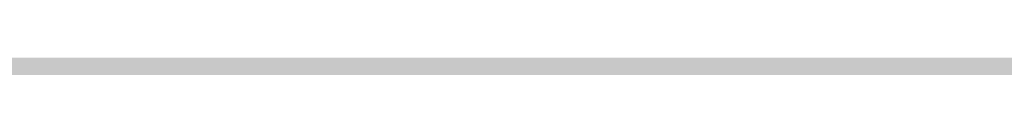
# Model space of a CAD drawing. Units: millimetres. Extents: x 0 to 2267, y 0 to 1823.
# Tile 106 of 256: x 1600.369 to 1605.705, y 1232.196 to 1232.23. Entities that reach past the tile are written whole.
import ezdxf

# ---------------------------------------------------------------- set-up
doc = ezdxf.new("R2010")
doc.units = ezdxf.units.MM
doc.header["$MEASUREMENT"] = 0
doc.layers.add('M-DIMS', color=2, linetype='Continuous', lineweight=25)
doc.layers.add('M-HATC', color=252, linetype='Continuous', lineweight=18)
doc.styles.get("Standard").update_dxf_attribs({"font": 'arial.ttf'})
doc.dimstyles.get("Standard").update_dxf_attribs({"dimtxt": 7, "dimasz": 4, "dimexe": 0.18, "dimexo": 0.0625, "dimgap": 0.09, "dimtad": 0, "dimdec": 0, "dimzin": 0, "dimdsep": 46, "dimtxsty": 'Standard', "dimcen": 0.09, "dimadec": 0, "dimazin": 0, "dimtfac": 1, "dimtdec": 0, "dimtofl": 0, "dimtmove": 0, "dimatfit": 3, "dimfxl": 1, "dimtolj": 1, "dimtzin": 0, "dimarcsym": 0})

# ---------------------------------------------------------------- blocks, each defined once
blk = doc.blocks.new('*D19')
at = {"layer": 'Defpoints', "color": 0, "transparency": 16777216}
for p in [(1605.3399, 1483.3044), (1445.5291, 1333.8851)]:
    blk.add_point(p, dxfattribs=at)
at = {"layer": 'M-DIMS', "color": 0, "lineweight": -2, "transparency": 16777216}
for p, q in [((1605.3399, 1483.2144), (1605.3399, 1483.3944)), ((1605.2499, 1483.3044), (1605.4299, 1483.3044)), ((1366.3244, 1259.8306), (1442.6072, 1331.1532))]:
    blk.add_line(p, q, dxfattribs=at)
at = {"layer": 'M-DIMS', "color": 0, "transparency": 16777216}
blk.add_solid([(1442.1519, 1331.6402), (1443.0625, 1330.6663), (1445.5291, 1333.8851)], dxfattribs=at)
at = {"layer": 'M-DIMS', "color": 0, "transparency": 16777216, "insert": (1349.6425, 1244.2335), "char_height": 7, "attachment_point": 5, "rotation": 43.0753}
blk.add_mtext('\\A1;2X R218.8', dxfattribs=at)

msp = doc.modelspace()

# ---------------------------------------------------------------- hatches: boundary and pattern name
at = {"layer": 'M-HATC'}
h = msp.add_hatch(color=256, dxfattribs=at)
h.dxf.hatch_style = 1
h.paths.add_polyline_path([(2055.771, 1603.062), (1381.0868, 1603.062), (1381.0868, 1598.062), (2055.771, 1598.062)])
h.paths.add_polyline_path([(2055.771, 1598.062), (1381.0868, 1598.062), (1381.0868, 1593.062), (2055.771, 1593.062)])
h.paths.add_polyline_path([(2051.3074, 1536.7609), (1385.5504, 1536.7609), (1385.5504, 1526.7609), (1387.5504, 1526.7609), (1388.5366, 1525.0528), (1385.3319, 1521.2335), (1385.3319, 1521.2226), (2050.2542, 1522.7491), (2048.3212, 1525.0528), (2049.3074, 1526.7609), (2051.3074, 1526.7609)])
edge = h.paths.add_edge_path()
edge.add_arc((1847.5345, 1379.1492), 135, 222.603061, 222.890851, ccw=False)
edge.add_line((1748.1663, 1287.7656), (1683.0921, 1287.7656))
edge.add_arc((1583.7239, 1379.1492), 135, 317.109149, 317.396939, ccw=False)
edge.add_arc((1678.9686, 1290.6707), 5, 222.8909, 317.1091, ccw=False)
edge.add_arc((1774.2133, 1379.1492), 135, 222.603061, 222.890851, ccw=False)
edge.add_line((1674.8451, 1287.7656), (1609.7709, 1287.7656))
edge.add_arc((1510.4027, 1379.1492), 135, 317.109149, 317.396939, ccw=False)
edge.add_arc((1605.6474, 1290.6707), 5, 222.8909, 317.1091, ccw=False)
edge.add_arc((1700.8921, 1379.1492), 135, 222.603061, 222.890851, ccw=False)
edge.add_line((1601.5239, 1287.7656), (1536.4497, 1287.7656))
edge.add_arc((1437.0815, 1379.1492), 135, 317.109149, 317.396939, ccw=False)
edge.add_arc((1532.3262, 1290.6707), 5, 222.8909, 317.1091, ccw=False)
edge.add_arc((1627.5709, 1379.1492), 135, 222.603061, 222.890851, ccw=False)
edge.add_line((1528.2027, 1287.7656), (1505.9289, 1287.7656))
edge.add_spline(control_points=[(1505.9289, 1287.7656), (1504.2622, 1287.7656), (1504.2622, 1282.7656), (1505.9289, 1282.7656)], knot_values=[0, 0, 0, 0, 5, 5, 5, 5], degree=3, periodic=0)
edge.add_line((1505.9289, 1282.7656), (1930.9289, 1282.7656))
edge.add_spline(control_points=[(1930.9289, 1282.7656), (1932.5956, 1282.7656), (1932.5956, 1287.7656), (1930.9289, 1287.7656)], knot_values=[0, 0, 0, 0, 5, 5, 5, 5], degree=3, periodic=0)
edge.add_line((1930.9289, 1287.7656), (1903.0557, 1287.7656))
edge.add_arc((1803.6875, 1379.1492), 135, 317.109149, 317.396939, ccw=False)
edge.add_arc((1898.9322, 1290.6707), 5, 222.8909, 317.1091, ccw=False)
edge.add_arc((1994.1769, 1379.1492), 135, 222.603061, 222.890851, ccw=False)
edge.add_line((1894.8087, 1287.7656), (1829.7345, 1287.7656))
edge.add_arc((1730.3663, 1379.1492), 135, 317.109149, 317.396939, ccw=False)
edge.add_arc((1825.611, 1290.6707), 5, 222.8909, 317.1091, ccw=False)
edge.add_arc((1920.8557, 1379.1492), 135, 222.603061, 222.890851, ccw=False)
edge.add_line((1821.4875, 1287.7656), (1756.4133, 1287.7656))
edge.add_arc((1657.0451, 1379.1492), 135, 317.109149, 317.396939, ccw=False)
edge.add_arc((1752.2898, 1290.6707), 5, 222.8909, 317.1091, ccw=False)
edge = h.paths.add_edge_path()
edge.add_spline(control_points=[(1843.4289, 1227.2475), (1845.0956, 1227.2475), (1845.0956, 1232.2475), (1843.4289, 1232.2475)], knot_values=[0, 0, 0, 0, 5, 5, 5, 5], degree=3, periodic=0)
edge.add_line((1843.4289, 1232.2475), (1593.4289, 1232.2475))
edge.add_spline(control_points=[(1593.4289, 1232.2475), (1591.7622, 1232.2475), (1591.7622, 1227.2475), (1593.4289, 1227.2475)], knot_values=[0, 0, 0, 0, 5, 5, 5, 5], degree=3, periodic=0)
edge.add_line((1593.4289, 1227.2475), (1843.4289, 1227.2475))
h.paths.add_polyline_path([(1905.9289, 1127.4171), (1530.9289, 1127.4171, 0.414214), (1520.9289, 1117.4171), (1530.9289, 1117.4171), (1915.9289, 1117.4171, 0.414214)])
edge = h.paths.add_edge_path()
edge.add_arc((1397.0858, 1498.4078), 12.7299, 90.78215, 190.87871, ccw=False)
edge.add_line((1396.912, 1511.1365), (1428.0097, 1511.3488))
edge.add_line((1428.0097, 1511.3488), (1433.0097, 1511.3488))
edge.add_line((1433.0097, 1511.3488), (1434.439, 1511.3488))
edge.add_arc((1419.474, 1498.0804), 20, 41.561, 74.08211)
edge.add_line((1424.9592, 1517.3135), (1399.9351, 1517.2561))
edge.add_spline(control_points=[(1399.9307, 1517.2561), (1399.884, 1517.2131), (1399.8328, 1517.1689), (1399.7774, 1517.1236)], knot_values=[11.567499, 11.567499, 11.567499, 11.567499, 11.814249, 11.814249, 11.814249, 11.814249], degree=3, periodic=0)
edge.add_spline(control_points=[(1399.6328, 1517.0099), (1399.5831, 1516.9721), (1399.5307, 1516.9338), (1399.4759, 1516.8947)], knot_values=[11.167718, 11.167718, 11.167718, 11.167718, 11.365188, 11.365188, 11.365188, 11.365188], degree=3, periodic=0)
edge.add_spline(control_points=[(1399.3398, 1516.8001), (1399.1514, 1516.6719), (1398.9384, 1516.5377), (1398.704, 1516.3994)], knot_values=[10.376405, 10.376405, 10.376405, 10.376405, 11.00994, 11.00994, 11.00994, 11.00994], degree=3, periodic=0)
edge.add_spline(control_points=[(1398.6572, 1516.3719), (1398.5789, 1516.326), (1398.4983, 1516.2797), (1398.4155, 1516.2331)], knot_values=[10.125175, 10.125175, 10.125175, 10.125175, 10.334406, 10.334406, 10.334406, 10.334406], degree=3, periodic=0)
edge.add_spline(control_points=[(1398.2642, 1516.1487), (1398.196, 1516.1111), (1398.1263, 1516.0732), (1398.0555, 1516.0351)], knot_values=[9.832246, 9.832246, 9.832246, 9.832246, 9.999658, 9.999658, 9.999658, 9.999658], degree=3, periodic=0)
edge.add_spline(control_points=[(1397.9987, 1516.0048), (1397.7312, 1515.8621), (1397.446, 1515.7171), (1397.1466, 1515.5714)], knot_values=[9.161808, 9.161808, 9.161808, 9.161808, 9.787769, 9.787769, 9.787769, 9.787769], degree=3, periodic=0)
edge.add_spline(control_points=[(1397.1466, 1515.5714), (1396.8418, 1515.423), (1396.5222, 1515.274), (1396.1914, 1515.1262)], knot_values=[8.524455, 8.524455, 8.524455, 8.524455, 9.161808, 9.161808, 9.161808, 9.161808], degree=3, periodic=0)
edge.add_spline(control_points=[(1396.0777, 1515.0756), (1395.9854, 1515.0348), (1395.8922, 1514.994), (1395.7983, 1514.9534)], knot_values=[8.275193, 8.275193, 8.275193, 8.275193, 8.451726, 8.451726, 8.451726, 8.451726], degree=3, periodic=0)
edge.add_spline(control_points=[(1395.6018, 1514.8691), (1395.4997, 1514.8257), (1395.3968, 1514.7824), (1395.2932, 1514.7394)], knot_values=[7.962917, 7.962917, 7.962917, 7.962917, 8.152764, 8.152764, 8.152764, 8.152764], degree=3, periodic=0)
edge.add_spline(control_points=[(1395.2116, 1514.7057), (1394.8278, 1514.5475), (1394.4345, 1514.3929), (1394.0364, 1514.2442)], knot_values=[7.21254, 7.21254, 7.21254, 7.21254, 7.913148, 7.913148, 7.913148, 7.913148], degree=3, periodic=0)
edge.add_spline(control_points=[(1394.0364, 1514.2442), (1393.7076, 1514.1214), (1393.3754, 1514.0027), (1393.0427, 1513.8895)], knot_values=[6.633733, 6.633733, 6.633733, 6.633733, 7.21254, 7.21254, 7.21254, 7.21254], degree=3, periodic=0)
edge.add_spline(control_points=[(1392.8214, 1513.815), (1392.7198, 1513.7812), (1392.6181, 1513.7479), (1392.5166, 1513.7152)], knot_values=[6.328796, 6.328796, 6.328796, 6.328796, 6.505493, 6.505493, 6.505493, 6.505493], degree=3, periodic=0)
edge.add_spline(control_points=[(1392.5166, 1513.7152), (1392.3187, 1513.6515), (1392.1212, 1513.59), (1391.9244, 1513.531)], knot_values=[5.984605, 5.984605, 5.984605, 5.984605, 6.328796, 6.328796, 6.328796, 6.328796], degree=3, periodic=0)
edge.add_spline(control_points=[(1391.7915, 1513.4915), (1391.3122, 1513.3501), (1390.8384, 1513.2239), (1390.3784, 1513.1171)], knot_values=[5.066697, 5.066697, 5.066697, 5.066697, 5.907055, 5.907055, 5.907055, 5.907055], degree=3, periodic=0)
edge.add_spline(control_points=[(1390.3784, 1513.1171), (1390.1797, 1513.071), (1389.9836, 1513.0284), (1389.7907, 1512.9899)], knot_values=[4.70367, 4.70367, 4.70367, 4.70367, 5.066695, 5.066695, 5.066695, 5.066695], degree=3, periodic=0)
edge.add_spline(control_points=[(1389.422, 1512.9204), (1389.2459, 1512.8892), (1389.0729, 1512.8617), (1388.9036, 1512.8381)], knot_values=[4.130571, 4.130571, 4.130571, 4.130571, 4.469816, 4.469816, 4.469816, 4.469816], degree=3, periodic=0)
edge.add_spline(control_points=[(1388.9036, 1512.8381), (1388.591, 1512.7946), (1388.2911, 1512.7644), (1388.0071, 1512.7494)], knot_values=[3.504031, 3.504031, 3.504031, 3.504031, 4.130571, 4.130571, 4.130571, 4.130571], degree=3, periodic=0)
edge.add_spline(control_points=[(1387.9356, 1512.7459), (1387.8538, 1512.7423), (1387.7733, 1512.74), (1387.6944, 1512.739)], knot_values=[3.268866, 3.268866, 3.268866, 3.268866, 3.451164, 3.451164, 3.451164, 3.451164], degree=3, periodic=0)
edge.add_spline(control_points=[(1387.3351, 1512.7443), (1387.2076, 1512.7499), (1387.0847, 1512.7597), (1386.967, 1512.7739)], knot_values=[2.670686, 2.670686, 2.670686, 2.670686, 2.984, 2.984, 2.984, 2.984], degree=3, periodic=0)
edge.add_spline(control_points=[(1386.8327, 1512.7922), (1386.8209, 1512.7941), (1386.8092, 1512.7959), (1386.7975, 1512.7979)], knot_values=[2.516981, 2.516981, 2.516981, 2.516981, 2.549528, 2.549528, 2.549528, 2.549528], degree=3, periodic=0)
edge.add_spline(control_points=[(1386.4526, 1512.8735), (1386.4257, 1512.881), (1386.3993, 1512.889), (1386.3733, 1512.8972)], knot_values=[2.095869, 2.095869, 2.095869, 2.095869, 2.17941, 2.17941, 2.17941, 2.17941], degree=3, periodic=0)
edge.add_spline(control_points=[(1386.0691, 1513.0189), (1386.0634, 1513.0217), (1386.0577, 1513.0246), (1386.052, 1513.0275)], knot_values=[1.72453, 1.72453, 1.72453, 1.72453, 1.745933, 1.745933, 1.745933, 1.745933], degree=3, periodic=0)
edge.add_arc((1399.474, 1498.0804), 20, 131.82432, 180)
edge.add_arc((1630.3336, 1505.5484), 250.9708, 181.705176, 236.427975)
edge.add_arc((1605.3399, 1483.3044), 218.7822, 238.660829, 243.34961)
edge.add_arc((1647.0911, 1510.3592), 262.8986, 183.129836, 237.853442, ccw=False)
h.paths.add_polyline_path([(1406.5369, 1391.9644, 0.149382), (1491.5506, 1296.4418, -0.129517)], flags=17)
edge = h.paths.add_edge_path()
edge.add_arc((2037.3838, 1498.0804), 20, 0, 48.26587)
edge.add_spline(control_points=[(2050.6973, 1513.0052), (2050.6512, 1512.9847), (2050.6034, 1512.9655), (2050.5539, 1512.9477)], knot_values=[1.835652, 1.835652, 1.835652, 1.835652, 2.000781, 2.000781, 2.000781, 2.000781], degree=3, periodic=0)
edge.add_spline(control_points=[(2050.4616, 1512.9166), (2050.479, 1512.9221), (2050.4963, 1512.9277), (2050.5133, 1512.9335)], knot_values=[2.045477, 2.045477, 2.045477, 2.045477, 2.101389, 2.101389, 2.101389, 2.101389], degree=3, periodic=0)
edge.add_spline(control_points=[(2050.129, 1512.8342), (2050.1984, 1512.8473), (2050.2657, 1512.8623), (2050.3308, 1512.8792)], knot_values=[2.237629, 2.237629, 2.237629, 2.237629, 2.435841, 2.435841, 2.435841, 2.435841], degree=3, periodic=0)
edge.add_spline(control_points=[(2050.0946, 1512.8278), (2050.1061, 1512.8299), (2050.1176, 1512.832), (2050.129, 1512.8342)], knot_values=[2.435841, 2.435841, 2.435841, 2.435841, 2.468321, 2.468321, 2.468321, 2.468321], degree=3, periodic=0)
edge.add_spline(control_points=[(2049.7843, 1512.7851), (2049.8552, 1512.7922), (2049.9243, 1512.8008), (2049.9917, 1512.8109)], knot_values=[2.563852, 2.563852, 2.563852, 2.563852, 2.748541, 2.748541, 2.748541, 2.748541], degree=3, periodic=0)
edge.add_spline(control_points=[(2049.4052, 1512.7617), (2049.5364, 1512.7653), (2049.6629, 1512.773), (2049.7843, 1512.7851)], knot_values=[2.748541, 2.748541, 2.748541, 2.748541, 3.064882, 3.064882, 3.064882, 3.064882], degree=3, periodic=0)
edge.add_spline(control_points=[(2049.1698, 1512.7597), (2049.2336, 1512.7591), (2049.2965, 1512.7594), (2049.3584, 1512.7606)], knot_values=[3.102309, 3.102309, 3.102309, 3.102309, 3.2503, 3.2503, 3.2503, 3.2503], degree=3, periodic=0)
edge.add_spline(control_points=[(2048.8573, 1512.7691), (2048.9638, 1512.7638), (2049.068, 1512.7606), (2049.1698, 1512.7597)], knot_values=[3.2503, 3.2503, 3.2503, 3.2503, 3.486069, 3.486069, 3.486069, 3.486069], degree=3, periodic=0)
edge.add_spline(control_points=[(2048.6924, 1512.7789), (2048.3729, 1512.8009), (2048.0345, 1512.8411), (2047.6817, 1512.897)], knot_values=[3.606429, 3.606429, 3.606429, 3.606429, 4.2989, 4.2989, 4.2989, 4.2989], degree=3, periodic=0)
edge.add_spline(control_points=[(2047.6817, 1512.897), (2047.5458, 1512.9185), (2047.4077, 1512.9424), (2047.2678, 1512.9685)], knot_values=[4.2989, 4.2989, 4.2989, 4.2989, 4.565769, 4.565769, 4.565769, 4.565769], degree=3, periodic=0)
edge.add_spline(control_points=[(2047.2678, 1512.9685), (2047.1449, 1512.9914), (2047.0207, 1513.016), (2046.8951, 1513.0422)], knot_values=[4.565769, 4.565769, 4.565769, 4.565769, 4.799971, 4.799971, 4.799971, 4.799971], degree=3, periodic=0)
edge.add_spline(control_points=[(2046.8951, 1513.0422), (2046.5286, 1513.1188), (2046.1513, 1513.209), (2045.7676, 1513.3107)], knot_values=[4.799971, 4.799971, 4.799971, 4.799971, 5.483718, 5.483718, 5.483718, 5.483718], degree=3, periodic=0)
edge.add_spline(control_points=[(2045.7676, 1513.3107), (2045.3724, 1513.4154), (2044.9704, 1513.5322), (2044.5662, 1513.6588)], knot_values=[5.483718, 5.483718, 5.483718, 5.483718, 6.187866, 6.187866, 6.187866, 6.187866], degree=3, periodic=0)
edge.add_spline(control_points=[(2044.5662, 1513.6588), (2044.4149, 1513.7061), (2044.2633, 1513.7549), (2044.1116, 1513.8048)], knot_values=[6.187866, 6.187866, 6.187866, 6.187866, 6.451551, 6.451551, 6.451551, 6.451551], degree=3, periodic=0)
edge.add_spline(control_points=[(2044.1116, 1513.8048), (2043.9967, 1513.8427), (2043.8817, 1513.8813), (2043.7668, 1513.9205)], knot_values=[6.451551, 6.451551, 6.451551, 6.451551, 6.651434, 6.651434, 6.651434, 6.651434], degree=3, periodic=0)
edge.add_spline(control_points=[(2043.7668, 1513.9205), (2043.3716, 1514.0554), (2042.9774, 1514.1979), (2042.5886, 1514.3458)], knot_values=[6.651434, 6.651434, 6.651434, 6.651434, 7.338879, 7.338879, 7.338879, 7.338879], degree=3, periodic=0)
edge.add_spline(control_points=[(2042.5886, 1514.3458), (2042.1643, 1514.5071), (2041.7465, 1514.6749), (2041.3409, 1514.846)], knot_values=[7.338879, 7.338879, 7.338879, 7.338879, 8.089209, 8.089209, 8.089209, 8.089209], degree=3, periodic=0)
edge.add_spline(control_points=[(2041.3409, 1514.846), (2041.1028, 1514.9465), (2040.869, 1515.0481), (2040.6405, 1515.1502)], knot_values=[8.089209, 8.089209, 8.089209, 8.089209, 8.529587, 8.529587, 8.529587, 8.529587], degree=3, periodic=0)
edge.add_spline(control_points=[(2040.51, 1515.2089), (2040.0824, 1515.4022), (2039.6747, 1515.5971), (2039.295, 1515.7894)], knot_values=[8.613818, 8.613818, 8.613818, 8.613818, 9.44571, 9.44571, 9.44571, 9.44571], degree=3, periodic=0)
edge.add_spline(control_points=[(2039.295, 1515.7894), (2039.0618, 1515.9075), (2038.8391, 1516.0246), (2038.6288, 1516.1398)], knot_values=[9.44571, 9.44571, 9.44571, 9.44571, 9.956404, 9.956404, 9.956404, 9.956404], degree=3, periodic=0)
edge.add_spline(control_points=[(2038.6288, 1516.1398), (2038.5187, 1516.2001), (2038.4121, 1516.2598), (2038.309, 1516.3189)], knot_values=[9.956404, 9.956404, 9.956404, 9.956404, 10.223542, 10.223542, 10.223542, 10.223542], degree=3, periodic=0)
edge.add_spline(control_points=[(2038.309, 1516.3189), (2038.2138, 1516.3735), (2038.1216, 1516.4276), (2038.0328, 1516.481)], knot_values=[10.223542, 10.223542, 10.223542, 10.223542, 10.47051, 10.47051, 10.47051, 10.47051], degree=3, periodic=0)
edge.add_spline(control_points=[(2038.0328, 1516.481), (2037.7855, 1516.6296), (2037.5639, 1516.773), (2037.3722, 1516.909)], knot_values=[10.47051, 10.47051, 10.47051, 10.47051, 11.15767, 11.15767, 11.15767, 11.15767], degree=3, periodic=0)
edge.add_spline(control_points=[(2037.3722, 1516.909), (2037.2789, 1516.9752), (2037.1927, 1517.0396), (2037.1142, 1517.102)], knot_values=[11.15767, 11.15767, 11.15767, 11.15767, 11.49227, 11.49227, 11.49227, 11.49227], degree=3, periodic=0)
edge.add_spline(control_points=[(2036.8564, 1517.3259), (2036.9148, 1517.2692), (2036.9814, 1517.2103), (2037.0557, 1517.1492)], knot_values=[11.577341, 11.577341, 11.577341, 11.577341, 11.91035, 11.91035, 11.91035, 11.91035], degree=3, periodic=0)
edge.add_spline(control_points=[(2036.8074, 1517.3748), (2036.823, 1517.3587), (2036.8393, 1517.3424), (2036.8564, 1517.3259)], knot_values=[11.91035, 11.91035, 11.91035, 11.91035, 12.007402, 12.007402, 12.007402, 12.007402], degree=3, periodic=0)
edge.add_spline(control_points=[(2036.7017, 1517.494), (2036.7104, 1517.483), (2036.7196, 1517.4719), (2036.7291, 1517.4606)], knot_values=[12.184155, 12.184155, 12.184155, 12.184155, 12.255409, 12.255409, 12.255409, 12.255409], degree=3, periodic=0)
edge.add_spline(control_points=[(2036.6159, 1517.6205), (2036.62, 1517.613), (2036.6243, 1517.6055), (2036.6289, 1517.5979)], knot_values=[12.487913, 12.487913, 12.487913, 12.487913, 12.541035, 12.541035, 12.541035, 12.541035], degree=3, periodic=0)
edge.add_spline(control_points=[(2036.5635, 1517.786), (2036.5637, 1517.7794), (2036.5642, 1517.7726), (2036.565, 1517.7658)], knot_values=[12.911761, 12.911761, 12.911761, 12.911761, 12.968286, 12.968286, 12.968286, 12.968286], degree=3, periodic=0)
edge.add_spline(control_points=[(2036.6166, 1517.9304), (2036.6125, 1517.9259), (2036.6086, 1517.9212), (2036.6049, 1517.9165)], knot_values=[13.382527, 13.382527, 13.382527, 13.382527, 13.433791, 13.433791, 13.433791, 13.433791], degree=3, periodic=0)
edge.add_spline(control_points=[(2036.749, 1518.017), (2036.7361, 1518.0116), (2036.7239, 1518.006), (2036.7124, 1518.0002)], knot_values=[13.726299, 13.726299, 13.726299, 13.726299, 13.809928, 13.809928, 13.809928, 13.809928], degree=3, periodic=0)
edge.add_spline(control_points=[(2036.8604, 1518.0528), (2036.8386, 1518.0474), (2036.8181, 1518.0416), (2036.7988, 1518.0353)], knot_values=[13.910887, 13.910887, 13.910887, 13.910887, 14.02153, 14.02153, 14.02153, 14.02153], degree=3, periodic=0)
edge.add_line((2036.9639, 1518.0804), (2032.3838, 1518.0804))
edge.add_line((2032.3838, 1518.0804), (2027.3838, 1518.0804))
edge.add_line((2027.3838, 1518.0804), (2022.3838, 1518.0804))
edge.add_line((2022.3838, 1518.0804), (2017.3838, 1518.0804))
edge.add_arc((2017.3838, 1498.0804), 20, 90, 138.439)
edge.add_line((2002.4188, 1511.3488), (2003.8481, 1511.3488))
edge.add_line((2003.8481, 1511.3488), (2008.8481, 1511.3488))
edge.add_line((2008.8481, 1511.3488), (2039.772, 1511.1377))
edge.add_arc((2039.772, 1498.4078), 12.7299, -10.87871, 90, ccw=False)
edge.add_arc((1789.7668, 1510.3592), 262.8986, 302.146558, 356.870164, ccw=False)
edge.add_arc((1831.5179, 1483.3044), 218.7822, 296.65039, 301.339171)
edge.add_arc((1806.5242, 1505.5484), 250.9708, 303.572025, 358.294824)
h.paths.add_polyline_path([(2030.321, 1391.9644, -0.129517), (1945.3072, 1296.4418, 0.149382)], flags=17)
edge = h.paths.add_edge_path()
edge.add_spline(control_points=[(2037.2464, 1518.0821), (2037.2898, 1518.081), (2037.3355, 1518.0804), (2037.3838, 1518.0804)], knot_values=[0.000012, 0.000012, 0.000012, 0.000012, 0.144754, 0.144754, 0.144754, 0.144754], degree=3, periodic=0)
edge.add_line((2037.3357, 1518.0804), (2037.0096, 1518.0804))
edge.add_spline(control_points=[(2037.0096, 1518.0804), (2036.9822, 1518.0768), (2036.956, 1518.0727), (2036.9312, 1518.0681)], knot_values=[14.13465, 14.13465, 14.13465, 14.13465, 14.247197, 14.247197, 14.247197, 14.247197], degree=3, periodic=0)
edge.add_spline(control_points=[(2036.9312, 1518.0681), (2036.9276, 1518.0674), (2036.9241, 1518.0667), (2036.9205, 1518.0661)], knot_values=[14.118315, 14.118315, 14.118315, 14.118315, 14.13465, 14.13465, 14.13465, 14.13465], degree=3, periodic=0)
edge.add_spline(control_points=[(2036.9205, 1518.0661), (2036.9118, 1518.0644), (2036.9032, 1518.0626), (2036.8948, 1518.0608)], knot_values=[14.078086, 14.078086, 14.078086, 14.078086, 14.118315, 14.118315, 14.118315, 14.118315], degree=3, periodic=0)
edge.add_spline(control_points=[(2036.8948, 1518.0608), (2036.883, 1518.0583), (2036.8716, 1518.0556), (2036.8604, 1518.0528)], knot_values=[14.02153, 14.02153, 14.02153, 14.02153, 14.078086, 14.078086, 14.078086, 14.078086], degree=3, periodic=0)
edge.add_spline(control_points=[(2036.8604, 1518.0528), (2036.8386, 1518.0474), (2036.8181, 1518.0416), (2036.7988, 1518.0353)], knot_values=[13.910887, 13.910887, 13.910887, 13.910887, 14.02153, 14.02153, 14.02153, 14.02153], degree=3, periodic=0)
edge.add_spline(control_points=[(2036.7988, 1518.0353), (2036.7981, 1518.035), (2036.7974, 1518.0348), (2036.7967, 1518.0346)], knot_values=[13.906906, 13.906906, 13.906906, 13.906906, 13.910887, 13.910887, 13.910887, 13.910887], degree=3, periodic=0)
edge.add_spline(control_points=[(2036.7967, 1518.0346), (2036.7882, 1518.0318), (2036.7799, 1518.0289), (2036.7719, 1518.0259)], knot_values=[13.857826, 13.857826, 13.857826, 13.857826, 13.906906, 13.906906, 13.906906, 13.906906], degree=3, periodic=0)
edge.add_spline(control_points=[(2036.7719, 1518.0259), (2036.764, 1518.023), (2036.7564, 1518.02), (2036.749, 1518.017)], knot_values=[13.809928, 13.809928, 13.809928, 13.809928, 13.857826, 13.857826, 13.857826, 13.857826], degree=3, periodic=0)
edge.add_spline(control_points=[(2036.749, 1518.017), (2036.7361, 1518.0116), (2036.7239, 1518.006), (2036.7124, 1518.0002)], knot_values=[13.726299, 13.726299, 13.726299, 13.726299, 13.809928, 13.809928, 13.809928, 13.809928], degree=3, periodic=0)
edge.add_spline(control_points=[(2036.7124, 1518.0002), (2036.7121, 1518), (2036.7118, 1517.9999), (2036.7115, 1517.9997)], knot_values=[13.723993, 13.723993, 13.723993, 13.723993, 13.726299, 13.726299, 13.726299, 13.726299], degree=3, periodic=0)
edge.add_spline(control_points=[(2036.7115, 1517.9997), (2036.7063, 1517.9971), (2036.7013, 1517.9944), (2036.6965, 1517.9917)], knot_values=[13.686536, 13.686536, 13.686536, 13.686536, 13.723993, 13.723993, 13.723993, 13.723993], degree=3, periodic=0)
edge.add_spline(control_points=[(2036.6965, 1517.9917), (2036.6919, 1517.9891), (2036.6874, 1517.9865), (2036.6831, 1517.9839)], knot_values=[13.651251, 13.651251, 13.651251, 13.651251, 13.686536, 13.686536, 13.686536, 13.686536], degree=3, periodic=0)
edge.add_spline(control_points=[(2036.6831, 1517.9839), (2036.6764, 1517.9798), (2036.67, 1517.9757), (2036.6639, 1517.9714)], knot_values=[13.596804, 13.596804, 13.596804, 13.596804, 13.651251, 13.651251, 13.651251, 13.651251], degree=3, periodic=0)
edge.add_spline(control_points=[(2036.6639, 1517.9714), (2036.6636, 1517.9712), (2036.6633, 1517.9709), (2036.6629, 1517.9707)], knot_values=[13.593956, 13.593956, 13.593956, 13.593956, 13.596804, 13.596804, 13.596804, 13.596804], degree=3, periodic=0)
edge.add_spline(control_points=[(2036.6629, 1517.9707), (2036.6603, 1517.9689), (2036.6577, 1517.967), (2036.6552, 1517.9651)], knot_values=[13.570322, 13.570322, 13.570322, 13.570322, 13.593956, 13.593956, 13.593956, 13.593956], degree=3, periodic=0)
edge.add_spline(control_points=[(2036.6552, 1517.9651), (2036.6525, 1517.9631), (2036.6499, 1517.9611), (2036.6474, 1517.9591)], knot_values=[13.545477, 13.545477, 13.545477, 13.545477, 13.570322, 13.570322, 13.570322, 13.570322], degree=3, periodic=0)
edge.add_spline(control_points=[(2036.6474, 1517.9591), (2036.6472, 1517.9589), (2036.6471, 1517.9588), (2036.6469, 1517.9587)], knot_values=[13.543931, 13.543931, 13.543931, 13.543931, 13.545477, 13.545477, 13.545477, 13.545477], degree=3, periodic=0)
edge.add_spline(control_points=[(2036.6469, 1517.9587), (2036.6412, 1517.9541), (2036.6358, 1517.9494), (2036.6307, 1517.9447)], knot_values=[13.488237, 13.488237, 13.488237, 13.488237, 13.543931, 13.543931, 13.543931, 13.543931], degree=3, periodic=0)
edge.add_spline(control_points=[(2036.6307, 1517.9447), (2036.6282, 1517.9423), (2036.6257, 1517.9399), (2036.6233, 1517.9374)], knot_values=[13.460307, 13.460307, 13.460307, 13.460307, 13.488237, 13.488237, 13.488237, 13.488237], degree=3, periodic=0)
edge.add_spline(control_points=[(2036.6233, 1517.9374), (2036.6215, 1517.9356), (2036.6198, 1517.9338), (2036.6181, 1517.932)], knot_values=[13.439712, 13.439712, 13.439712, 13.439712, 13.460307, 13.460307, 13.460307, 13.460307], degree=3, periodic=0)
edge.add_spline(control_points=[(2036.6181, 1517.932), (2036.6176, 1517.9315), (2036.6171, 1517.9309), (2036.6166, 1517.9304)], knot_values=[13.433791, 13.433791, 13.433791, 13.433791, 13.439712, 13.439712, 13.439712, 13.439712], degree=3, periodic=0)
edge.add_spline(control_points=[(2036.6166, 1517.9304), (2036.6125, 1517.9259), (2036.6086, 1517.9212), (2036.6049, 1517.9165)], knot_values=[13.382527, 13.382527, 13.382527, 13.382527, 13.433791, 13.433791, 13.433791, 13.433791], degree=3, periodic=0)
edge.add_spline(control_points=[(2036.6049, 1517.9165), (2036.6026, 1517.9135), (2036.6004, 1517.9104), (2036.5982, 1517.9074)], knot_values=[13.350017, 13.350017, 13.350017, 13.350017, 13.382527, 13.382527, 13.382527, 13.382527], degree=3, periodic=0)
edge.add_spline(control_points=[(2036.5982, 1517.9074), (2036.5972, 1517.9059), (2036.5962, 1517.9043), (2036.5952, 1517.9028)], knot_values=[13.333922, 13.333922, 13.333922, 13.333922, 13.350017, 13.350017, 13.350017, 13.350017], degree=3, periodic=0)
edge.add_spline(control_points=[(2036.5952, 1517.9028), (2036.5945, 1517.9018), (2036.5939, 1517.9009), (2036.5933, 1517.8999)], knot_values=[13.323828, 13.323828, 13.323828, 13.323828, 13.333922, 13.333922, 13.333922, 13.333922], degree=3, periodic=0)
edge.add_spline(control_points=[(2036.5933, 1517.8999), (2036.5905, 1517.8955), (2036.5879, 1517.8909), (2036.5855, 1517.8864)], knot_values=[13.277545, 13.277545, 13.277545, 13.277545, 13.323828, 13.323828, 13.323828, 13.323828], degree=3, periodic=0)
edge.add_spline(control_points=[(2036.5855, 1517.8864), (2036.5836, 1517.8827), (2036.5817, 1517.8789), (2036.5801, 1517.8751)], knot_values=[13.240119, 13.240119, 13.240119, 13.240119, 13.277545, 13.277545, 13.277545, 13.277545], degree=3, periodic=0)
edge.add_spline(control_points=[(2036.5801, 1517.8751), (2036.5795, 1517.8739), (2036.579, 1517.8727), (2036.5785, 1517.8715)], knot_values=[13.228211, 13.228211, 13.228211, 13.228211, 13.240119, 13.240119, 13.240119, 13.240119], degree=3, periodic=0)
edge.add_spline(control_points=[(2036.5785, 1517.8715), (2036.578, 1517.8702), (2036.5774, 1517.869), (2036.5769, 1517.8677)], knot_values=[13.215717, 13.215717, 13.215717, 13.215717, 13.228211, 13.228211, 13.228211, 13.228211], degree=3, periodic=0)
edge.add_spline(control_points=[(2036.5769, 1517.8677), (2036.5755, 1517.864), (2036.5741, 1517.8603), (2036.5729, 1517.8565)], knot_values=[13.179847, 13.179847, 13.179847, 13.179847, 13.215717, 13.215717, 13.215717, 13.215717], degree=3, periodic=0)
edge.add_spline(control_points=[(2036.5729, 1517.8565), (2036.5713, 1517.8515), (2036.5699, 1517.8464), (2036.5687, 1517.8413)], knot_values=[13.132017, 13.132017, 13.132017, 13.132017, 13.179847, 13.179847, 13.179847, 13.179847], degree=3, periodic=0)
edge.add_spline(control_points=[(2036.5687, 1517.8413), (2036.5684, 1517.8402), (2036.5682, 1517.8392), (2036.568, 1517.8382)], knot_values=[13.122482, 13.122482, 13.122482, 13.122482, 13.132017, 13.132017, 13.132017, 13.132017], degree=3, periodic=0)
edge.add_spline(control_points=[(2036.568, 1517.8382), (2036.5676, 1517.8363), (2036.5672, 1517.8345), (2036.5669, 1517.8327)], knot_values=[13.105592, 13.105592, 13.105592, 13.105592, 13.122482, 13.122482, 13.122482, 13.122482], degree=3, periodic=0)
edge.add_spline(control_points=[(2036.5669, 1517.8327), (2036.5662, 1517.8292), (2036.5657, 1517.8257), (2036.5652, 1517.8222)], knot_values=[13.074063, 13.074063, 13.074063, 13.074063, 13.105592, 13.105592, 13.105592, 13.105592], degree=3, periodic=0)
edge.add_spline(control_points=[(2036.5652, 1517.8222), (2036.5652, 1517.8222), (2036.5652, 1517.8222), (2036.5652, 1517.8222)], knot_values=[13.074043, 13.074043, 13.074043, 13.074043, 13.074063, 13.074063, 13.074063, 13.074063], degree=3, periodic=0)
edge.add_spline(control_points=[(2036.5652, 1517.8222), (2036.5644, 1517.8164), (2036.5639, 1517.8106), (2036.5636, 1517.8046)], knot_values=[13.021884, 13.021884, 13.021884, 13.021884, 13.074043, 13.074043, 13.074043, 13.074043], degree=3, periodic=0)
edge.add_spline(control_points=[(2036.5636, 1517.8046), (2036.5636, 1517.804), (2036.5636, 1517.8034), (2036.5635, 1517.8028)], knot_values=[13.01674, 13.01674, 13.01674, 13.01674, 13.021884, 13.021884, 13.021884, 13.021884], degree=3, periodic=0)
edge.add_spline(control_points=[(2036.5635, 1517.8028), (2036.5634, 1517.8005), (2036.5634, 1517.7982), (2036.5634, 1517.7958)], knot_values=[12.996438, 12.996438, 12.996438, 12.996438, 13.01674, 13.01674, 13.01674, 13.01674], degree=3, periodic=0)
edge.add_spline(control_points=[(2036.5634, 1517.7958), (2036.5633, 1517.7926), (2036.5634, 1517.7893), (2036.5635, 1517.786)], knot_values=[12.968286, 12.968286, 12.968286, 12.968286, 12.996438, 12.996438, 12.996438, 12.996438], degree=3, periodic=0)
edge.add_spline(control_points=[(2036.5635, 1517.786), (2036.5637, 1517.7794), (2036.5642, 1517.7726), (2036.565, 1517.7658)], knot_values=[12.911761, 12.911761, 12.911761, 12.911761, 12.968286, 12.968286, 12.968286, 12.968286], degree=3, periodic=0)
edge.add_spline(control_points=[(2036.565, 1517.7658), (2036.565, 1517.7657), (2036.565, 1517.7656), (2036.565, 1517.7656)], knot_values=[12.911017, 12.911017, 12.911017, 12.911017, 12.911761, 12.911761, 12.911761, 12.911761], degree=3, periodic=0)
edge.add_spline(control_points=[(2036.565, 1517.7656), (2036.5654, 1517.7625), (2036.5658, 1517.7593), (2036.5663, 1517.7562)], knot_values=[12.88528, 12.88528, 12.88528, 12.88528, 12.911017, 12.911017, 12.911017, 12.911017], degree=3, periodic=0)
edge.add_spline(control_points=[(2036.5663, 1517.7562), (2036.5667, 1517.7534), (2036.5672, 1517.7506), (2036.5677, 1517.7478)], knot_values=[12.862519, 12.862519, 12.862519, 12.862519, 12.88528, 12.88528, 12.88528, 12.88528], degree=3, periodic=0)
edge.add_spline(control_points=[(2036.5677, 1517.7478), (2036.5678, 1517.7474), (2036.5679, 1517.7469), (2036.568, 1517.7465)], knot_values=[12.858885, 12.858885, 12.858885, 12.858885, 12.862519, 12.862519, 12.862519, 12.862519], degree=3, periodic=0)
edge.add_spline(control_points=[(2036.568, 1517.7465), (2036.5692, 1517.7399), (2036.5707, 1517.7332), (2036.5724, 1517.7264)], knot_values=[12.8053, 12.8053, 12.8053, 12.8053, 12.858885, 12.858885, 12.858885, 12.858885], degree=3, periodic=0)
edge.add_spline(control_points=[(2036.5724, 1517.7264), (2036.5734, 1517.7226), (2036.5745, 1517.7187), (2036.5756, 1517.7149)], knot_values=[12.775176, 12.775176, 12.775176, 12.775176, 12.8053, 12.8053, 12.8053, 12.8053], degree=3, periodic=0)
edge.add_spline(control_points=[(2036.5756, 1517.7149), (2036.5763, 1517.7125), (2036.577, 1517.7102), (2036.5778, 1517.7078)], knot_values=[12.756759, 12.756759, 12.756759, 12.756759, 12.775176, 12.775176, 12.775176, 12.775176], degree=3, periodic=0)
edge.add_spline(control_points=[(2036.5778, 1517.7078), (2036.5781, 1517.7067), (2036.5784, 1517.7057), (2036.5787, 1517.7047)], knot_values=[12.748742, 12.748742, 12.748742, 12.748742, 12.756759, 12.756759, 12.756759, 12.756759], degree=3, periodic=0)
edge.add_spline(control_points=[(2036.5787, 1517.7047), (2036.5808, 1517.6983), (2036.5831, 1517.6919), (2036.5856, 1517.6854)], knot_values=[12.69959, 12.69959, 12.69959, 12.69959, 12.748742, 12.748742, 12.748742, 12.748742], degree=3, periodic=0)
edge.add_spline(control_points=[(2036.5856, 1517.6854), (2036.5876, 1517.68), (2036.5898, 1517.6746), (2036.5921, 1517.6692)], knot_values=[12.659038, 12.659038, 12.659038, 12.659038, 12.69959, 12.69959, 12.69959, 12.69959], degree=3, periodic=0)
edge.add_spline(control_points=[(2036.5921, 1517.6692), (2036.594, 1517.6648), (2036.5959, 1517.6605), (2036.5979, 1517.6561)], knot_values=[12.626806, 12.626806, 12.626806, 12.626806, 12.659038, 12.659038, 12.659038, 12.659038], degree=3, periodic=0)
edge.add_spline(control_points=[(2036.5979, 1517.6561), (2036.5984, 1517.6551), (2036.5989, 1517.6541), (2036.5993, 1517.6531)], knot_values=[12.619394, 12.619394, 12.619394, 12.619394, 12.626806, 12.626806, 12.626806, 12.626806], degree=3, periodic=0)
edge.add_spline(control_points=[(2036.5993, 1517.6531), (2036.6043, 1517.6424), (2036.6099, 1517.6315), (2036.6159, 1517.6205)], knot_values=[12.541039, 12.541039, 12.541039, 12.541039, 12.619394, 12.619394, 12.619394, 12.619394], degree=3, periodic=0)
edge.add_spline(control_points=[(2036.6159, 1517.6205), (2036.6159, 1517.6205), (2036.6159, 1517.6205), (2036.6159, 1517.6205)], knot_values=[12.541035, 12.541035, 12.541035, 12.541035, 12.541039, 12.541039, 12.541039, 12.541039], degree=3, periodic=0)
edge.add_spline(control_points=[(2036.6159, 1517.6205), (2036.62, 1517.613), (2036.6243, 1517.6055), (2036.6289, 1517.5979)], knot_values=[12.487913, 12.487913, 12.487913, 12.487913, 12.541035, 12.541035, 12.541035, 12.541035], degree=3, periodic=0)
edge.add_spline(control_points=[(2036.6289, 1517.5979), (2036.6326, 1517.5916), (2036.6365, 1517.5853), (2036.6406, 1517.5789)], knot_values=[12.443982, 12.443982, 12.443982, 12.443982, 12.487913, 12.487913, 12.487913, 12.487913], degree=3, periodic=0)
edge.add_spline(control_points=[(2036.6406, 1517.5789), (2036.6414, 1517.5776), (2036.6423, 1517.5763), (2036.6431, 1517.5749)], knot_values=[12.434996, 12.434996, 12.434996, 12.434996, 12.443982, 12.443982, 12.443982, 12.443982], degree=3, periodic=0)
edge.add_spline(control_points=[(2036.6431, 1517.5749), (2036.6531, 1517.5596), (2036.6639, 1517.5439), (2036.6756, 1517.528)], knot_values=[12.329647, 12.329647, 12.329647, 12.329647, 12.434996, 12.434996, 12.434996, 12.434996], degree=3, periodic=0)
edge.add_spline(control_points=[(2036.6756, 1517.528), (2036.6839, 1517.5168), (2036.6925, 1517.5055), (2036.7017, 1517.494)], knot_values=[12.255409, 12.255409, 12.255409, 12.255409, 12.329647, 12.329647, 12.329647, 12.329647], degree=3, periodic=0)
edge.add_spline(control_points=[(2036.7017, 1517.494), (2036.7104, 1517.483), (2036.7196, 1517.4719), (2036.7291, 1517.4606)], knot_values=[12.184155, 12.184155, 12.184155, 12.184155, 12.255409, 12.255409, 12.255409, 12.255409], degree=3, periodic=0)
edge.add_spline(control_points=[(2036.7291, 1517.4606), (2036.7436, 1517.4435), (2036.759, 1517.4262), (2036.7753, 1517.4085)], knot_values=[12.075961, 12.075961, 12.075961, 12.075961, 12.184155, 12.184155, 12.184155, 12.184155], degree=3, periodic=0)
edge.add_spline(control_points=[(2036.7753, 1517.4085), (2036.7763, 1517.4075), (2036.7773, 1517.4064), (2036.7783, 1517.4054)], knot_values=[12.069502, 12.069502, 12.069502, 12.069502, 12.075961, 12.075961, 12.075961, 12.075961], degree=3, periodic=0)
edge.add_spline(control_points=[(2036.7783, 1517.4054), (2036.7877, 1517.3953), (2036.7974, 1517.385), (2036.8074, 1517.3748)], knot_values=[12.007402, 12.007402, 12.007402, 12.007402, 12.069502, 12.069502, 12.069502, 12.069502], degree=3, periodic=0)
edge.add_spline(control_points=[(2036.8074, 1517.3748), (2036.823, 1517.3587), (2036.8393, 1517.3424), (2036.8564, 1517.3259)], knot_values=[11.91035, 11.91035, 11.91035, 11.91035, 12.007402, 12.007402, 12.007402, 12.007402], degree=3, periodic=0)
edge.add_spline(control_points=[(2036.8564, 1517.3259), (2036.9148, 1517.2692), (2036.9814, 1517.2103), (2037.0557, 1517.1492)], knot_values=[11.577341, 11.577341, 11.577341, 11.577341, 11.91035, 11.91035, 11.91035, 11.91035], degree=3, periodic=0)
edge.add_spline(control_points=[(2037.0557, 1517.1492), (2037.0747, 1517.1336), (2037.0942, 1517.1179), (2037.1142, 1517.102)], knot_values=[11.49227, 11.49227, 11.49227, 11.49227, 11.577341, 11.577341, 11.577341, 11.577341], degree=3, periodic=0)
edge.add_spline(control_points=[(2037.1142, 1517.102), (2037.1927, 1517.0396), (2037.2789, 1516.9752), (2037.3722, 1516.909)], knot_values=[11.15767, 11.15767, 11.15767, 11.15767, 11.49227, 11.49227, 11.49227, 11.49227], degree=3, periodic=0)
edge.add_spline(control_points=[(2037.3722, 1516.909), (2037.5639, 1516.773), (2037.7855, 1516.6296), (2038.0328, 1516.481)], knot_values=[10.47051, 10.47051, 10.47051, 10.47051, 11.15767, 11.15767, 11.15767, 11.15767], degree=3, periodic=0)
edge.add_spline(control_points=[(2038.0328, 1516.481), (2038.1216, 1516.4276), (2038.2138, 1516.3735), (2038.309, 1516.3189)], knot_values=[10.223542, 10.223542, 10.223542, 10.223542, 10.47051, 10.47051, 10.47051, 10.47051], degree=3, periodic=0)
edge.add_spline(control_points=[(2038.309, 1516.3189), (2038.4121, 1516.2598), (2038.5187, 1516.2001), (2038.6288, 1516.1398)], knot_values=[9.956404, 9.956404, 9.956404, 9.956404, 10.223542, 10.223542, 10.223542, 10.223542], degree=3, periodic=0)
edge.add_spline(control_points=[(2038.6288, 1516.1398), (2038.8391, 1516.0246), (2039.0618, 1515.9075), (2039.295, 1515.7894)], knot_values=[9.44571, 9.44571, 9.44571, 9.44571, 9.956404, 9.956404, 9.956404, 9.956404], degree=3, periodic=0)
edge.add_spline(control_points=[(2039.295, 1515.7894), (2039.6747, 1515.5971), (2040.0824, 1515.4022), (2040.51, 1515.2089)], knot_values=[8.613818, 8.613818, 8.613818, 8.613818, 9.44571, 9.44571, 9.44571, 9.44571], degree=3, periodic=0)
edge.add_spline(control_points=[(2040.51, 1515.2089), (2040.5533, 1515.1893), (2040.5968, 1515.1697), (2040.6405, 1515.1502)], knot_values=[8.529587, 8.529587, 8.529587, 8.529587, 8.613818, 8.613818, 8.613818, 8.613818], degree=3, periodic=0)
edge.add_spline(control_points=[(2040.6405, 1515.1502), (2040.869, 1515.0481), (2041.1028, 1514.9465), (2041.3409, 1514.846)], knot_values=[8.089209, 8.089209, 8.089209, 8.089209, 8.529587, 8.529587, 8.529587, 8.529587], degree=3, periodic=0)
edge.add_spline(control_points=[(2041.3409, 1514.846), (2041.7465, 1514.6749), (2042.1643, 1514.5071), (2042.5886, 1514.3458)], knot_values=[7.338879, 7.338879, 7.338879, 7.338879, 8.089209, 8.089209, 8.089209, 8.089209], degree=3, periodic=0)
edge.add_spline(control_points=[(2042.5886, 1514.3458), (2042.9774, 1514.1979), (2043.3716, 1514.0554), (2043.7668, 1513.9205)], knot_values=[6.651434, 6.651434, 6.651434, 6.651434, 7.338879, 7.338879, 7.338879, 7.338879], degree=3, periodic=0)
edge.add_spline(control_points=[(2043.7668, 1513.9205), (2043.8817, 1513.8813), (2043.9967, 1513.8427), (2044.1116, 1513.8048)], knot_values=[6.451551, 6.451551, 6.451551, 6.451551, 6.651434, 6.651434, 6.651434, 6.651434], degree=3, periodic=0)
edge.add_spline(control_points=[(2044.1116, 1513.8048), (2044.2633, 1513.7549), (2044.4149, 1513.7061), (2044.5662, 1513.6588)], knot_values=[6.187866, 6.187866, 6.187866, 6.187866, 6.451551, 6.451551, 6.451551, 6.451551], degree=3, periodic=0)
edge.add_spline(control_points=[(2044.5662, 1513.6588), (2044.9704, 1513.5322), (2045.3724, 1513.4154), (2045.7676, 1513.3107)], knot_values=[5.483718, 5.483718, 5.483718, 5.483718, 6.187866, 6.187866, 6.187866, 6.187866], degree=3, periodic=0)
edge.add_spline(control_points=[(2045.7676, 1513.3107), (2046.1513, 1513.209), (2046.5286, 1513.1188), (2046.8951, 1513.0422)], knot_values=[4.799971, 4.799971, 4.799971, 4.799971, 5.483718, 5.483718, 5.483718, 5.483718], degree=3, periodic=0)
edge.add_spline(control_points=[(2046.8951, 1513.0422), (2047.0207, 1513.016), (2047.1449, 1512.9914), (2047.2678, 1512.9685)], knot_values=[4.565769, 4.565769, 4.565769, 4.565769, 4.799971, 4.799971, 4.799971, 4.799971], degree=3, periodic=0)
edge.add_spline(control_points=[(2047.2678, 1512.9685), (2047.4077, 1512.9424), (2047.5458, 1512.9185), (2047.6817, 1512.897)], knot_values=[4.2989, 4.2989, 4.2989, 4.2989, 4.565769, 4.565769, 4.565769, 4.565769], degree=3, periodic=0)
edge.add_spline(control_points=[(2047.6817, 1512.897), (2048.0345, 1512.8411), (2048.3729, 1512.8009), (2048.6924, 1512.7789)], knot_values=[3.606429, 3.606429, 3.606429, 3.606429, 4.2989, 4.2989, 4.2989, 4.2989], degree=3, periodic=0)
edge.add_spline(control_points=[(2048.6924, 1512.7789), (2048.7479, 1512.7751), (2048.8029, 1512.7718), (2048.8573, 1512.7691)], knot_values=[3.486069, 3.486069, 3.486069, 3.486069, 3.606429, 3.606429, 3.606429, 3.606429], degree=3, periodic=0)
edge.add_spline(control_points=[(2048.8573, 1512.7691), (2048.9638, 1512.7638), (2049.068, 1512.7606), (2049.1698, 1512.7597)], knot_values=[3.2503, 3.2503, 3.2503, 3.2503, 3.486069, 3.486069, 3.486069, 3.486069], degree=3, periodic=0)
edge.add_spline(control_points=[(2049.1698, 1512.7597), (2049.2336, 1512.7591), (2049.2965, 1512.7594), (2049.3584, 1512.7606)], knot_values=[3.102309, 3.102309, 3.102309, 3.102309, 3.2503, 3.2503, 3.2503, 3.2503], degree=3, periodic=0)
edge.add_spline(control_points=[(2049.3584, 1512.7606), (2049.3741, 1512.7609), (2049.3897, 1512.7613), (2049.4052, 1512.7617)], knot_values=[3.064882, 3.064882, 3.064882, 3.064882, 3.102309, 3.102309, 3.102309, 3.102309], degree=3, periodic=0)
edge.add_spline(control_points=[(2049.4052, 1512.7617), (2049.5364, 1512.7653), (2049.6629, 1512.773), (2049.7843, 1512.7851)], knot_values=[2.748541, 2.748541, 2.748541, 2.748541, 3.064882, 3.064882, 3.064882, 3.064882], degree=3, periodic=0)
edge.add_spline(control_points=[(2049.7843, 1512.7851), (2049.8552, 1512.7922), (2049.9243, 1512.8008), (2049.9917, 1512.8109)], knot_values=[2.563852, 2.563852, 2.563852, 2.563852, 2.748541, 2.748541, 2.748541, 2.748541], degree=3, periodic=0)
edge.add_spline(control_points=[(2049.9917, 1512.8109), (2050.0265, 1512.8161), (2050.0608, 1512.8218), (2050.0946, 1512.8278)], knot_values=[2.468321, 2.468321, 2.468321, 2.468321, 2.563852, 2.563852, 2.563852, 2.563852], degree=3, periodic=0)
edge.add_spline(control_points=[(2050.0946, 1512.8278), (2050.1061, 1512.8299), (2050.1176, 1512.832), (2050.129, 1512.8342)], knot_values=[2.435841, 2.435841, 2.435841, 2.435841, 2.468321, 2.468321, 2.468321, 2.468321], degree=3, periodic=0)
edge.add_spline(control_points=[(2050.129, 1512.8342), (2050.1984, 1512.8473), (2050.2657, 1512.8623), (2050.3308, 1512.8792)], knot_values=[2.237629, 2.237629, 2.237629, 2.237629, 2.435841, 2.435841, 2.435841, 2.435841], degree=3, periodic=0)
edge.add_spline(control_points=[(2050.3308, 1512.8792), (2050.3754, 1512.8908), (2050.4191, 1512.9032), (2050.4616, 1512.9166)], knot_values=[2.101389, 2.101389, 2.101389, 2.101389, 2.237629, 2.237629, 2.237629, 2.237629], degree=3, periodic=0)
edge.add_spline(control_points=[(2050.4616, 1512.9166), (2050.479, 1512.9221), (2050.4963, 1512.9277), (2050.5133, 1512.9335)], knot_values=[2.045477, 2.045477, 2.045477, 2.045477, 2.101389, 2.101389, 2.101389, 2.101389], degree=3, periodic=0)
edge.add_spline(control_points=[(2050.5133, 1512.9335), (2050.527, 1512.9382), (2050.5405, 1512.9429), (2050.5539, 1512.9477)], knot_values=[2.000781, 2.000781, 2.000781, 2.000781, 2.045477, 2.045477, 2.045477, 2.045477], degree=3, periodic=0)
edge.add_spline(control_points=[(2050.5539, 1512.9477), (2050.6034, 1512.9655), (2050.6512, 1512.9847), (2050.6973, 1513.0052)], knot_values=[1.835652, 1.835652, 1.835652, 1.835652, 2.000781, 2.000781, 2.000781, 2.000781], degree=3, periodic=0)
edge.add_arc((2037.3838, 1498.0804), 20, 48.26587, 90.12993)
edge = h.paths.add_edge_path(flags=16)
edge.add_spline(control_points=[(1386.1389, 1512.9859), (1388.92, 1511.7395), (1398.0387, 1515.5187), (1399.9307, 1517.2561)], knot_values=[1.831046, 1.831046, 1.831046, 1.831046, 11.814249, 11.814249, 11.814249, 11.814249], degree=3, periodic=0)
edge.add_line((1399.9307, 1517.2561), (1393.7435, 1517.2419))
edge.add_arc((1399.474, 1498.0804), 20, 106.6501, 131.8173)

# ---------------------------------------------------------------- dimensions: what is measured, and where the dimension line sits
at = {"layer": 'M-DIMS'}
dim = msp.add_radius_dim(center=(1605.3399, 1483.3044), mpoint=(1445.5291, 1333.8851), text='2X <>', dimstyle='Standard', override={"dimdec": 1, "dimlfac": 1, "dimrnd": 0, "dimzin": 0, "dimdsep": 46, "dimlunit": 2}, dxfattribs=at)
dim.commit()
dim.dimension.update_dxf_attribs({"geometry": '*D19', "text_midpoint": (1349.6425, 1244.2335), "dimtype": 164})

doc.saveas('drawing.dxf')
